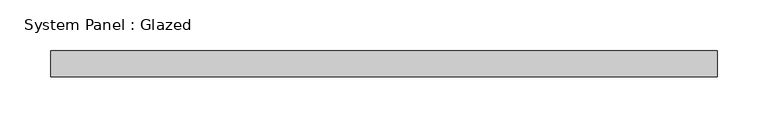
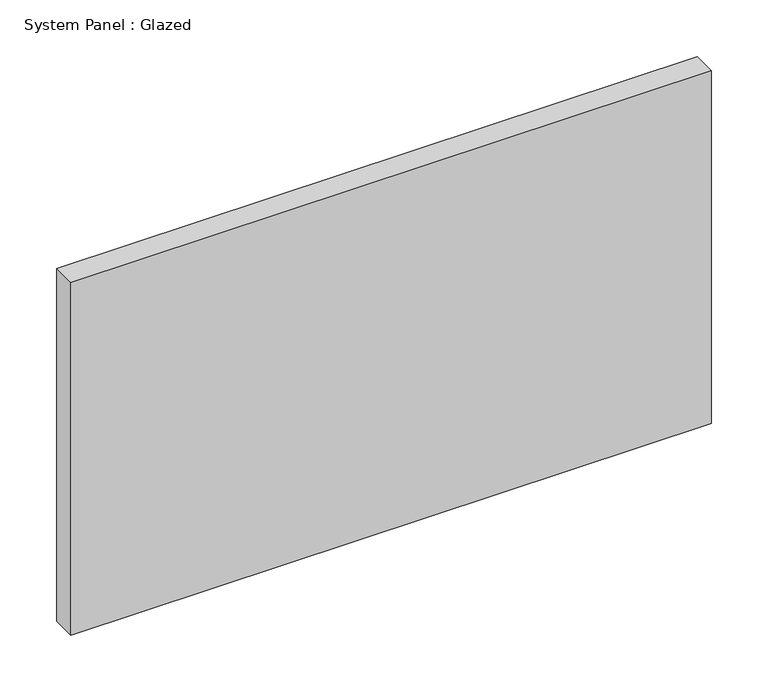
"""IFC4 building model written with IfcOpenShell, lengths in millimetres: plate geometry, System Panel : Glazed."""

from ifc_helpers import new_model, si_unit, origin, origin_with_axes, place, context, project, spatial, polyline, outline, extrude, source, transform, mapped, element, save


def system_panel_glazed_f5251298(model_context):
    return source(origin(), model_context, "Body", "SweptSolid", [
        extrude(outline(polyline([(327.025, 19.05), (-327.025, 19.05), (-327.025, 44.45), (327.025, 44.45), (327.025, 19.05)])), origin_with_axes(), (0.0, 0.0, 1.0), 381.0),
    ])


if __name__ == "__main__":
    model = new_model("IFC4")
    model_context = context("Model", 3, world=origin())
    ifc_project = project(units=[si_unit("LENGTHUNIT", "METRE", prefix="MILLI")], contexts=[model_context])
    site = spatial("IfcSite", under=ifc_project)
    building = spatial("IfcBuilding", under=site)
    placement = place(None, origin())
    system_panel_glazed_shape = system_panel_glazed_f5251298(model_context)
    element("IfcPlate", 1, ObjectType="System Panel : Glazed", at=placement, inside=building, context=model_context, shape_type="MappedRepresentation", body=[
        mapped(system_panel_glazed_shape, transform((0.0, 0.0, 0.0), x_axis=(1.0, 0.0, 0.0), y_axis=(0.0, 1.0, 0.0), z_axis=(0.0, 0.0, 1.0))),
    ])
    save(model, "model.ifc")

# Revit data of these elements
# Type "System Panel : Glazed"
#   Construction Type Id = "GSP4R"
#   Analytic Construction = "1/8 in Pilkington single glazing"
#   Visual Light Transmittance = 0.9
#   Solar Heat Gain Coefficient = 0.86
#   Heat Transfer Coefficient (U) = 1.18115 BTU/(h·ft²·°F)
#   Define Thermal Properties by = 1
# Element 1 (IfcPlate, "System Panel : Glazed")
#   Materials on its faces: "Glass"
# Materials
#   "Glass": class "Glass", colour RGB 0 128 192, transparency 0.75, Description = "Soda Lime Glass", Cost = 0
